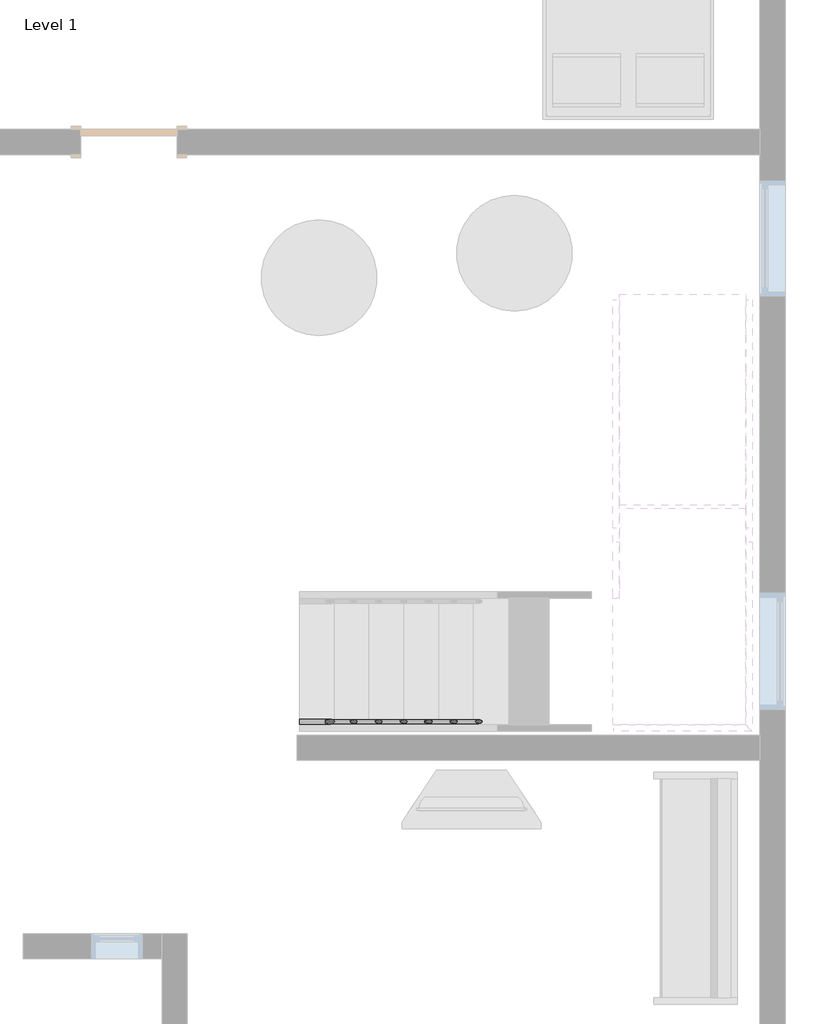
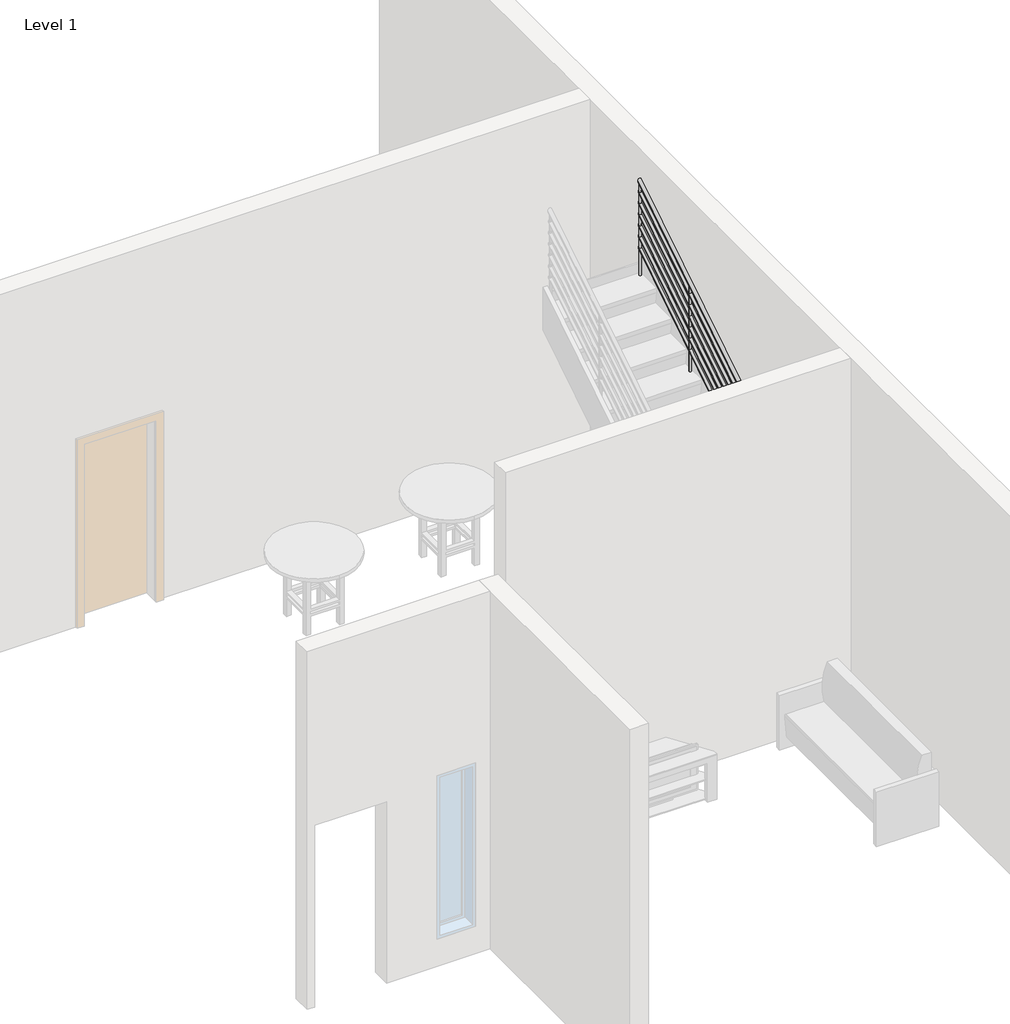
# One storey, part 3 of 4: 1 railing.
"""IFC4 building model written with IfcOpenShell, lengths in millimetres."""

from ifc_helpers import new_model, si_unit, point, frame, frame_2d, origin, place, context, project, spatial, circle_curve, ellipse_curve, trimmed, segment, composite_curve, outline, extrude, element, save
from ifc_brep_helpers import plane_surface, cylinder_surface, advanced_brep

model = new_model("IFC4")

# Units and contexts
model_context = context("Model", 3, world=origin())
ifc_project = project(units=[si_unit("LENGTHUNIT", "METRE", prefix="MILLI")], contexts=[model_context])

# Site, building, storey
site = spatial("IfcSite", under=ifc_project)
building = spatial("IfcBuilding", under=site)
storey = spatial("IfcBuildingStorey", under=building, Name="Level 1", Elevation=0.0)

# Railing
placement = place(None, origin())
element("IfcRailing", 1, ObjectType="900mm Pipe", at=placement, inside=storey, context=model_context, shape_type="SolidModel", body=[
    advanced_brep(
    [(-399.786154, 2752.4262668, 1050.2491997), (-399.786154, 2792.4262668, 1050.2491997), (2081.007299, 2752.4262668, 2619.1304348), (2081.007299, 2792.4262668, 2619.1304348), (3120.6396272, 2752.4262668, 2619.1304348), (3080.6396272, 2792.4262668, 2619.1304348), (3120.6396272, 4184.041917, 2619.1304348), (3080.6396272, 4184.041917, 2619.1304348), (3120.6396272, 6103.248464, 3832.8578953), (3080.6396272, 6103.248464, 3832.8578953)],
    [
        (0, 1, ellipse_curve(frame((-399.786154, 2772.4262668, 1050.2491997), z_axis=(-1.0, 0.0, 0.0), x_axis=(0.0, 0.0, -1.0)), 23.6638438, 20.0)),
        (1, 0, ellipse_curve(frame((-399.786154, 2772.4262668, 1050.2491997), z_axis=(-1.0, 0.0, 0.0), x_axis=(0.0, 0.0, -1.0)), 23.6638438, 20.0)),
        (0, 2),
        (2, 3, ellipse_curve(frame((2081.007299, 2772.4262668, 2619.1304348), z_axis=(-0.9605132043335073, 0.0, -0.2782344053149758), x_axis=(0.2782344053149764, 0.0, -0.9605132043335071)), 20.822202, 20.0)),
        (3, 1),
        (3, 2, ellipse_curve(frame((2081.007299, 2772.4262668, 2619.1304348), z_axis=(-0.9605132043335073, 0.0, -0.2782344053149758), x_axis=(0.2782344053149764, 0.0, -0.9605132043335071)), 20.822202, 20.0)),
        (2, 4),
        (4, 5, ellipse_curve(frame((3100.6396272, 2772.4262668, 2619.1304348), z_axis=(-0.7071067811865493, -0.7071067811865456, 0.0), x_axis=(-0.7071067811865458, 0.7071067811865492, 0.0)), 28.2842712, 20.0)),
        (5, 3),
        (5, 4, ellipse_curve(frame((3100.6396272, 2772.4262668, 2619.1304348), z_axis=(-0.7071067811865493, -0.7071067811865456, 0.0), x_axis=(-0.7071067811865458, 0.7071067811865492, 0.0)), 28.2842712, 20.0)),
        (4, 6),
        (6, 7, ellipse_curve(frame((3100.6396272, 4184.041917, 2619.1304348), z_axis=(0.0, -0.9605132043335073, -0.27823440531497556), x_axis=(0.0, -0.27823440531497573, 0.9605132043335072)), 20.822202, 20.0)),
        (7, 5),
        (7, 6, ellipse_curve(frame((3100.6396272, 4184.041917, 2619.1304348), z_axis=(0.0, -0.9605132043335073, -0.27823440531497556), x_axis=(0.0, -0.27823440531497573, 0.9605132043335072)), 20.822202, 20.0)),
        (8, 9, ellipse_curve(frame((3100.6396272, 6103.248464, 3832.8578953), z_axis=(0.0, 1.0, 0.0), x_axis=(0.0, 0.0, -1.0)), 23.6638438, 20.0)),
        (9, 8, ellipse_curve(frame((3100.6396272, 6103.248464, 3832.8578953), z_axis=(0.0, 1.0, 0.0), x_axis=(0.0, 0.0, -1.0)), 23.6638438, 20.0)),
        (6, 8),
        (9, 7),
    ],
    [
        plane_surface(frame((-399.786154, 2772.4262668, 1073.9130435), z_axis=(-1.0, 0.0, 0.0), x_axis=(0.0, 1.0, 0.0))),
        cylinder_surface(frame((-389.0962412, 2772.4262668, 1057.0096189), z_axis=(-0.8451712313980436, 0.0, -0.5344956404098303), x_axis=(0.0, 1.0, 0.0)), 20.0),
        cylinder_surface(frame((2075.213846, 2772.4262668, 2619.1304348), z_axis=(-1.0, 0.0, 0.0), x_axis=(0.0, 1.0, 0.0)), 20.0),
        cylinder_surface(frame((3100.6396272, 2772.4262668, 2619.1304348), z_axis=(0.0, -1.0, 0.0), x_axis=(-1.0, 0.0, 0.0)), 20.0),
        plane_surface(frame((3100.6396272, 6103.248464, 3856.5217391), z_axis=(0.0, 1.0, 0.0), x_axis=(0.0, 0.0, 1.0))),
        cylinder_surface(frame((3100.6396272, 4188.9383768, 2622.2270102), z_axis=(0.0, -0.8451712313980438, -0.5344956404098301), x_axis=(-1.0, 0.0, 0.0)), 20.0),
    ],
    [
        (0, [[1, 2]]),
        (1, [[-1, 3, 4, 5]]),
        (1, [[-2, -5, 6, -3]]),
        (2, [[-4, 7, 8, 9]]),
        (2, [[-6, -9, 10, -7]]),
        (3, [[-8, 11, 12, 13]]),
        (3, [[-10, -13, 14, -11]]),
        (4, [[15, 16]]),
        (5, [[-12, 17, -16, 18]]),
        (5, [[-14, -18, -15, -17]]),
    ],
),
    advanced_brep(
    [(-399.786154, 2787.4262668, 931.1651606), (-399.786154, 2757.4262668, 931.1651606), (2079.5589357, 2787.4262668, 2499.1304348), (2079.5589357, 2757.4262668, 2499.1304348), (3085.6396272, 2787.4262668, 2499.1304348), (3115.6396272, 2757.4262668, 2499.1304348), (3085.6396272, 4182.5935537, 2499.1304348), (3115.6396272, 4182.5935537, 2499.1304348), (3085.6396272, 6103.248464, 3713.7738563), (3115.6396272, 6103.248464, 3713.7738563)],
    [
        (0, 1, ellipse_curve(frame((-399.786154, 2772.4262668, 931.1651606), z_axis=(-1.0, 0.0, 0.0), x_axis=(0.0, 0.0, -1.0)), 17.7478828, 15.0)),
        (1, 0, ellipse_curve(frame((-399.786154, 2772.4262668, 931.1651606), z_axis=(-1.0, 0.0, 0.0), x_axis=(0.0, 0.0, -1.0)), 17.7478828, 15.0)),
        (0, 2),
        (2, 3, ellipse_curve(frame((2079.5589357, 2772.4262668, 2499.1304348), z_axis=(-0.9605132043335073, 0.0, -0.2782344053149758), x_axis=(0.2782344053149764, 0.0, -0.9605132043335071)), 15.6166515, 15.0)),
        (3, 1),
        (3, 2, ellipse_curve(frame((2079.5589357, 2772.4262668, 2499.1304348), z_axis=(-0.9605132043335073, 0.0, -0.2782344053149758), x_axis=(0.2782344053149764, 0.0, -0.9605132043335071)), 15.6166515, 15.0)),
        (2, 4),
        (4, 5, ellipse_curve(frame((3100.6396272, 2772.4262668, 2499.1304348), z_axis=(-0.7071067811865493, -0.7071067811865456, 0.0), x_axis=(-0.7071067811865458, 0.7071067811865492, 0.0)), 21.2132034, 15.0)),
        (5, 3),
        (5, 4, ellipse_curve(frame((3100.6396272, 2772.4262668, 2499.1304348), z_axis=(-0.7071067811865493, -0.7071067811865456, 0.0), x_axis=(-0.7071067811865458, 0.7071067811865492, 0.0)), 21.2132034, 15.0)),
        (4, 6),
        (6, 7, ellipse_curve(frame((3100.6396272, 4182.5935537, 2499.1304348), z_axis=(0.0, -0.9605132043335073, -0.27823440531497556), x_axis=(0.0, -0.27823440531497573, 0.9605132043335072)), 15.6166515, 15.0)),
        (7, 5),
        (7, 6, ellipse_curve(frame((3100.6396272, 4182.5935537, 2499.1304348), z_axis=(0.0, -0.9605132043335073, -0.27823440531497556), x_axis=(0.0, -0.27823440531497573, 0.9605132043335072)), 15.6166515, 15.0)),
        (8, 9, ellipse_curve(frame((3100.6396272, 6103.248464, 3713.7738563), z_axis=(0.0, 1.0, 0.0), x_axis=(0.0, 0.0, -1.0)), 17.7478828, 15.0)),
        (9, 8, ellipse_curve(frame((3100.6396272, 6103.248464, 3713.7738563), z_axis=(0.0, 1.0, 0.0), x_axis=(0.0, 0.0, -1.0)), 17.7478828, 15.0)),
        (6, 8),
        (9, 7),
    ],
    [
        plane_surface(frame((-399.786154, 2772.4262668, 948.9130435), z_axis=(-1.0, 0.0, 0.0), x_axis=(0.0, 1.0, 0.0))),
        cylinder_surface(frame((-391.7687194, 2772.4262668, 936.235475), z_axis=(-0.8451712313980436, 0.0, -0.5344956404098303), x_axis=(0.0, -1.0, 0.0)), 15.0),
        cylinder_surface(frame((2075.213846, 2772.4262668, 2499.1304348), z_axis=(-1.0, 0.0, 0.0), x_axis=(0.0, -1.0, 0.0)), 15.0),
        cylinder_surface(frame((3100.6396272, 2772.4262668, 2499.1304348), z_axis=(0.0, -1.0, 0.0), x_axis=(1.0, 0.0, 0.0)), 15.0),
        plane_surface(frame((3100.6396272, 6103.248464, 3731.5217391), z_axis=(0.0, 1.0, 0.0), x_axis=(0.0, 0.0, 1.0))),
        cylinder_surface(frame((3100.6396272, 4186.2658986, 2501.4528663), z_axis=(0.0, -0.8451712313980438, -0.5344956404098301), x_axis=(1.0, 0.0, 0.0)), 15.0),
    ],
    [
        (0, [[1, 2]]),
        (1, [[-1, 3, 4, 5]]),
        (1, [[-2, -5, 6, -3]]),
        (2, [[-4, 7, 8, 9]]),
        (2, [[-6, -9, 10, -7]]),
        (3, [[-8, 11, 12, 13]]),
        (3, [[-10, -13, 14, -11]]),
        (4, [[15, 16]]),
        (5, [[-12, 17, -16, 18]]),
        (5, [[-14, -18, -15, -17]]),
    ],
),
    advanced_brep(
    [(-399.786154, 2787.4262668, 806.1651606), (-399.786154, 2757.4262668, 806.1651606), (2079.5589357, 2787.4262668, 2374.1304348), (2079.5589357, 2757.4262668, 2374.1304348), (3085.6396272, 2787.4262668, 2374.1304348), (3115.6396272, 2757.4262668, 2374.1304348), (3085.6396272, 4182.5935537, 2374.1304348), (3115.6396272, 4182.5935537, 2374.1304348), (3085.6396272, 6103.248464, 3588.7738563), (3115.6396272, 6103.248464, 3588.7738563)],
    [
        (0, 1, ellipse_curve(frame((-399.786154, 2772.4262668, 806.1651606), z_axis=(-1.0, 0.0, 0.0), x_axis=(0.0, 0.0, -1.0)), 17.7478828, 15.0)),
        (1, 0, ellipse_curve(frame((-399.786154, 2772.4262668, 806.1651606), z_axis=(-1.0, 0.0, 0.0), x_axis=(0.0, 0.0, -1.0)), 17.7478828, 15.0)),
        (0, 2),
        (2, 3, ellipse_curve(frame((2079.5589357, 2772.4262668, 2374.1304348), z_axis=(-0.9605132043335073, 0.0, -0.2782344053149758), x_axis=(0.2782344053149764, 0.0, -0.9605132043335071)), 15.6166515, 15.0)),
        (3, 1),
        (3, 2, ellipse_curve(frame((2079.5589357, 2772.4262668, 2374.1304348), z_axis=(-0.9605132043335073, 0.0, -0.2782344053149758), x_axis=(0.2782344053149764, 0.0, -0.9605132043335071)), 15.6166515, 15.0)),
        (2, 4),
        (4, 5, ellipse_curve(frame((3100.6396272, 2772.4262668, 2374.1304348), z_axis=(-0.7071067811865493, -0.7071067811865456, 0.0), x_axis=(-0.7071067811865458, 0.7071067811865492, 0.0)), 21.2132034, 15.0)),
        (5, 3),
        (5, 4, ellipse_curve(frame((3100.6396272, 2772.4262668, 2374.1304348), z_axis=(-0.7071067811865493, -0.7071067811865456, 0.0), x_axis=(-0.7071067811865458, 0.7071067811865492, 0.0)), 21.2132034, 15.0)),
        (4, 6),
        (6, 7, ellipse_curve(frame((3100.6396272, 4182.5935537, 2374.1304348), z_axis=(0.0, -0.9605132043335073, -0.27823440531497556), x_axis=(0.0, -0.27823440531497573, 0.9605132043335072)), 15.6166515, 15.0)),
        (7, 5),
        (7, 6, ellipse_curve(frame((3100.6396272, 4182.5935537, 2374.1304348), z_axis=(0.0, -0.9605132043335073, -0.27823440531497556), x_axis=(0.0, -0.27823440531497573, 0.9605132043335072)), 15.6166515, 15.0)),
        (8, 9, ellipse_curve(frame((3100.6396272, 6103.248464, 3588.7738563), z_axis=(0.0, 1.0, 0.0), x_axis=(0.0, 0.0, -1.0)), 17.7478828, 15.0)),
        (9, 8, ellipse_curve(frame((3100.6396272, 6103.248464, 3588.7738563), z_axis=(0.0, 1.0, 0.0), x_axis=(0.0, 0.0, -1.0)), 17.7478828, 15.0)),
        (6, 8),
        (9, 7),
    ],
    [
        plane_surface(frame((-399.786154, 2772.4262668, 823.9130435), z_axis=(-1.0, 0.0, 0.0), x_axis=(0.0, 1.0, 0.0))),
        cylinder_surface(frame((-391.7687194, 2772.4262668, 811.235475), z_axis=(-0.8451712313980436, 0.0, -0.5344956404098303), x_axis=(0.0, -1.0, 0.0)), 15.0),
        cylinder_surface(frame((2075.213846, 2772.4262668, 2374.1304348), z_axis=(-1.0, 0.0, 0.0), x_axis=(0.0, -1.0, 0.0)), 15.0),
        cylinder_surface(frame((3100.6396272, 2772.4262668, 2374.1304348), z_axis=(0.0, -1.0, 0.0), x_axis=(1.0, 0.0, 0.0)), 15.0),
        plane_surface(frame((3100.6396272, 6103.248464, 3606.5217391), z_axis=(0.0, 1.0, 0.0), x_axis=(0.0, 0.0, 1.0))),
        cylinder_surface(frame((3100.6396272, 4186.2658986, 2376.4528663), z_axis=(0.0, -0.8451712313980438, -0.5344956404098301), x_axis=(1.0, 0.0, 0.0)), 15.0),
    ],
    [
        (0, [[1, 2]]),
        (1, [[-1, 3, 4, 5]]),
        (1, [[-2, -5, 6, -3]]),
        (2, [[-4, 7, 8, 9]]),
        (2, [[-6, -9, 10, -7]]),
        (3, [[-8, 11, 12, 13]]),
        (3, [[-10, -13, 14, -11]]),
        (4, [[15, 16]]),
        (5, [[-12, 17, -16, 18]]),
        (5, [[-14, -18, -15, -17]]),
    ],
),
    advanced_brep(
    [(-399.786154, 2787.4262668, 681.1651606), (-399.786154, 2757.4262668, 681.1651606), (2079.5589357, 2787.4262668, 2249.1304348), (2079.5589357, 2757.4262668, 2249.1304348), (3085.6396272, 2787.4262668, 2249.1304348), (3115.6396272, 2757.4262668, 2249.1304348), (3085.6396272, 4182.5935537, 2249.1304348), (3115.6396272, 4182.5935537, 2249.1304348), (3085.6396272, 6103.248464, 3463.7738563), (3115.6396272, 6103.248464, 3463.7738563)],
    [
        (0, 1, ellipse_curve(frame((-399.786154, 2772.4262668, 681.1651606), z_axis=(-1.0, 0.0, 0.0), x_axis=(0.0, 0.0, -1.0)), 17.7478828, 15.0)),
        (1, 0, ellipse_curve(frame((-399.786154, 2772.4262668, 681.1651606), z_axis=(-1.0, 0.0, 0.0), x_axis=(0.0, 0.0, -1.0)), 17.7478828, 15.0)),
        (0, 2),
        (2, 3, ellipse_curve(frame((2079.5589357, 2772.4262668, 2249.1304348), z_axis=(-0.9605132043335073, 0.0, -0.2782344053149758), x_axis=(0.2782344053149764, 0.0, -0.9605132043335071)), 15.6166515, 15.0)),
        (3, 1),
        (3, 2, ellipse_curve(frame((2079.5589357, 2772.4262668, 2249.1304348), z_axis=(-0.9605132043335073, 0.0, -0.2782344053149758), x_axis=(0.2782344053149764, 0.0, -0.9605132043335071)), 15.6166515, 15.0)),
        (2, 4),
        (4, 5, ellipse_curve(frame((3100.6396272, 2772.4262668, 2249.1304348), z_axis=(-0.7071067811865493, -0.7071067811865456, 0.0), x_axis=(-0.7071067811865458, 0.7071067811865492, 0.0)), 21.2132034, 15.0)),
        (5, 3),
        (5, 4, ellipse_curve(frame((3100.6396272, 2772.4262668, 2249.1304348), z_axis=(-0.7071067811865493, -0.7071067811865456, 0.0), x_axis=(-0.7071067811865458, 0.7071067811865492, 0.0)), 21.2132034, 15.0)),
        (4, 6),
        (6, 7, ellipse_curve(frame((3100.6396272, 4182.5935537, 2249.1304348), z_axis=(0.0, -0.9605132043335073, -0.27823440531497545), x_axis=(0.0, -0.27823440531497584, 0.9605132043335073)), 15.6166515, 15.0)),
        (7, 5),
        (7, 6, ellipse_curve(frame((3100.6396272, 4182.5935537, 2249.1304348), z_axis=(0.0, -0.9605132043335073, -0.27823440531497545), x_axis=(0.0, -0.27823440531497584, 0.9605132043335073)), 15.6166515, 15.0)),
        (8, 9, ellipse_curve(frame((3100.6396272, 6103.248464, 3463.7738563), z_axis=(0.0, 1.0, 0.0), x_axis=(0.0, 0.0, -1.0)), 17.7478828, 15.0)),
        (9, 8, ellipse_curve(frame((3100.6396272, 6103.248464, 3463.7738563), z_axis=(0.0, 1.0, 0.0), x_axis=(0.0, 0.0, -1.0)), 17.7478828, 15.0)),
        (6, 8),
        (9, 7),
    ],
    [
        plane_surface(frame((-399.786154, 2772.4262668, 698.9130435), z_axis=(-1.0, 0.0, 0.0), x_axis=(0.0, 1.0, 0.0))),
        cylinder_surface(frame((-391.7687194, 2772.4262668, 686.235475), z_axis=(-0.8451712313980436, 0.0, -0.5344956404098303), x_axis=(0.0, -1.0, 0.0)), 15.0),
        cylinder_surface(frame((2075.213846, 2772.4262668, 2249.1304348), z_axis=(-1.0, 0.0, 0.0), x_axis=(0.0, -1.0, 0.0)), 15.0),
        cylinder_surface(frame((3100.6396272, 2772.4262668, 2249.1304348), z_axis=(0.0, -1.0, 0.0), x_axis=(1.0, 0.0, 0.0)), 15.0),
        plane_surface(frame((3100.6396272, 6103.248464, 3481.5217391), z_axis=(0.0, 1.0, 0.0), x_axis=(0.0, 0.0, 1.0))),
        cylinder_surface(frame((3100.6396272, 4186.2658986, 2251.4528663), z_axis=(0.0, -0.845171231398044, -0.5344956404098299), x_axis=(1.0, 0.0, 0.0)), 15.0),
    ],
    [
        (0, [[1, 2]]),
        (1, [[-1, 3, 4, 5]]),
        (1, [[-2, -5, 6, -3]]),
        (2, [[-4, 7, 8, 9]]),
        (2, [[-6, -9, 10, -7]]),
        (3, [[-8, 11, 12, 13]]),
        (3, [[-10, -13, 14, -11]]),
        (4, [[15, 16]]),
        (5, [[-12, 17, -16, 18]]),
        (5, [[-14, -18, -15, -17]]),
    ],
),
    advanced_brep(
    [(-399.786154, 2787.4262668, 556.1651606), (-399.786154, 2757.4262668, 556.1651606), (2079.5589357, 2787.4262668, 2124.1304348), (2079.5589357, 2757.4262668, 2124.1304348), (3085.6396272, 2787.4262668, 2124.1304348), (3115.6396272, 2757.4262668, 2124.1304348), (3085.6396272, 4182.5935537, 2124.1304348), (3115.6396272, 4182.5935537, 2124.1304348), (3085.6396272, 6103.248464, 3338.7738563), (3115.6396272, 6103.248464, 3338.7738563)],
    [
        (0, 1, ellipse_curve(frame((-399.786154, 2772.4262668, 556.1651606), z_axis=(-1.0, 0.0, 0.0), x_axis=(0.0, 0.0, -1.0)), 17.7478828, 15.0)),
        (1, 0, ellipse_curve(frame((-399.786154, 2772.4262668, 556.1651606), z_axis=(-1.0, 0.0, 0.0), x_axis=(0.0, 0.0, -1.0)), 17.7478828, 15.0)),
        (0, 2),
        (2, 3, ellipse_curve(frame((2079.5589357, 2772.4262668, 2124.1304348), z_axis=(-0.9605132043335073, 0.0, -0.2782344053149758), x_axis=(0.2782344053149764, 0.0, -0.9605132043335071)), 15.6166515, 15.0)),
        (3, 1),
        (3, 2, ellipse_curve(frame((2079.5589357, 2772.4262668, 2124.1304348), z_axis=(-0.9605132043335073, 0.0, -0.2782344053149758), x_axis=(0.2782344053149764, 0.0, -0.9605132043335071)), 15.6166515, 15.0)),
        (2, 4),
        (4, 5, ellipse_curve(frame((3100.6396272, 2772.4262668, 2124.1304348), z_axis=(-0.7071067811865493, -0.7071067811865456, 0.0), x_axis=(-0.7071067811865458, 0.7071067811865492, 0.0)), 21.2132034, 15.0)),
        (5, 3),
        (5, 4, ellipse_curve(frame((3100.6396272, 2772.4262668, 2124.1304348), z_axis=(-0.7071067811865493, -0.7071067811865456, 0.0), x_axis=(-0.7071067811865458, 0.7071067811865492, 0.0)), 21.2132034, 15.0)),
        (4, 6),
        (6, 7, ellipse_curve(frame((3100.6396272, 4182.5935537, 2124.1304348), z_axis=(0.0, -0.9605132043335073, -0.27823440531497556), x_axis=(0.0, -0.27823440531497573, 0.9605132043335072)), 15.6166515, 15.0)),
        (7, 5),
        (7, 6, ellipse_curve(frame((3100.6396272, 4182.5935537, 2124.1304348), z_axis=(0.0, -0.9605132043335073, -0.27823440531497556), x_axis=(0.0, -0.27823440531497573, 0.9605132043335072)), 15.6166515, 15.0)),
        (8, 9, ellipse_curve(frame((3100.6396272, 6103.248464, 3338.7738563), z_axis=(0.0, 1.0, 0.0), x_axis=(0.0, 0.0, -1.0)), 17.7478828, 15.0)),
        (9, 8, ellipse_curve(frame((3100.6396272, 6103.248464, 3338.7738563), z_axis=(0.0, 1.0, 0.0), x_axis=(0.0, 0.0, -1.0)), 17.7478828, 15.0)),
        (6, 8),
        (9, 7),
    ],
    [
        plane_surface(frame((-399.786154, 2772.4262668, 573.9130435), z_axis=(-1.0, 0.0, 0.0), x_axis=(0.0, 1.0, 0.0))),
        cylinder_surface(frame((-391.7687194, 2772.4262668, 561.235475), z_axis=(-0.8451712313980436, 0.0, -0.5344956404098303), x_axis=(0.0, -1.0, 0.0)), 15.0),
        cylinder_surface(frame((2075.213846, 2772.4262668, 2124.1304348), z_axis=(-1.0, 0.0, 0.0), x_axis=(0.0, -1.0, 0.0)), 15.0),
        cylinder_surface(frame((3100.6396272, 2772.4262668, 2124.1304348), z_axis=(0.0, -1.0, 0.0), x_axis=(1.0, 0.0, 0.0)), 15.0),
        plane_surface(frame((3100.6396272, 6103.248464, 3356.5217391), z_axis=(0.0, 1.0, 0.0), x_axis=(0.0, 0.0, 1.0))),
        cylinder_surface(frame((3100.6396272, 4186.2658986, 2126.4528663), z_axis=(0.0, -0.8451712313980438, -0.5344956404098301), x_axis=(1.0, 0.0, 0.0)), 15.0),
    ],
    [
        (0, [[1, 2]]),
        (1, [[-1, 3, 4, 5]]),
        (1, [[-2, -5, 6, -3]]),
        (2, [[-4, 7, 8, 9]]),
        (2, [[-6, -9, 10, -7]]),
        (3, [[-8, 11, 12, 13]]),
        (3, [[-10, -13, 14, -11]]),
        (4, [[15, 16]]),
        (5, [[-12, 17, -16, 18]]),
        (5, [[-14, -18, -15, -17]]),
    ],
),
    advanced_brep(
    [(-399.786154, 2787.4262668, 431.1651606), (-399.786154, 2757.4262668, 431.1651606), (2079.5589357, 2787.4262668, 1999.1304348), (2079.5589357, 2757.4262668, 1999.1304348), (3085.6396272, 2787.4262668, 1999.1304348), (3115.6396272, 2757.4262668, 1999.1304348), (3085.6396272, 4182.5935537, 1999.1304348), (3115.6396272, 4182.5935537, 1999.1304348), (3085.6396272, 6103.248464, 3213.7738563), (3115.6396272, 6103.248464, 3213.7738563)],
    [
        (0, 1, ellipse_curve(frame((-399.786154, 2772.4262668, 431.1651606), z_axis=(-1.0, 0.0, 0.0), x_axis=(0.0, 0.0, -1.0)), 17.7478828, 15.0)),
        (1, 0, ellipse_curve(frame((-399.786154, 2772.4262668, 431.1651606), z_axis=(-1.0, 0.0, 0.0), x_axis=(0.0, 0.0, -1.0)), 17.7478828, 15.0)),
        (0, 2),
        (2, 3, ellipse_curve(frame((2079.5589357, 2772.4262668, 1999.1304348), z_axis=(-0.9605132043335073, 0.0, -0.2782344053149758), x_axis=(0.2782344053149764, 0.0, -0.9605132043335071)), 15.6166515, 15.0)),
        (3, 1),
        (3, 2, ellipse_curve(frame((2079.5589357, 2772.4262668, 1999.1304348), z_axis=(-0.9605132043335073, 0.0, -0.2782344053149758), x_axis=(0.2782344053149764, 0.0, -0.9605132043335071)), 15.6166515, 15.0)),
        (2, 4),
        (4, 5, ellipse_curve(frame((3100.6396272, 2772.4262668, 1999.1304348), z_axis=(-0.7071067811865493, -0.7071067811865456, 0.0), x_axis=(-0.7071067811865458, 0.7071067811865492, 0.0)), 21.2132034, 15.0)),
        (5, 3),
        (5, 4, ellipse_curve(frame((3100.6396272, 2772.4262668, 1999.1304348), z_axis=(-0.7071067811865493, -0.7071067811865456, 0.0), x_axis=(-0.7071067811865458, 0.7071067811865492, 0.0)), 21.2132034, 15.0)),
        (4, 6),
        (6, 7, ellipse_curve(frame((3100.6396272, 4182.5935537, 1999.1304348), z_axis=(0.0, -0.9605132043335072, -0.27823440531497556), x_axis=(0.0, -0.2782344053149761, 0.9605132043335072)), 15.6166515, 15.0)),
        (7, 5),
        (7, 6, ellipse_curve(frame((3100.6396272, 4182.5935537, 1999.1304348), z_axis=(0.0, -0.9605132043335072, -0.27823440531497556), x_axis=(0.0, -0.2782344053149761, 0.9605132043335072)), 15.6166515, 15.0)),
        (8, 9, ellipse_curve(frame((3100.6396272, 6103.248464, 3213.7738563), z_axis=(0.0, 1.0, 0.0), x_axis=(0.0, 0.0, -1.0)), 17.7478828, 15.0)),
        (9, 8, ellipse_curve(frame((3100.6396272, 6103.248464, 3213.7738563), z_axis=(0.0, 1.0, 0.0), x_axis=(0.0, 0.0, -1.0)), 17.7478828, 15.0)),
        (6, 8),
        (9, 7),
    ],
    [
        plane_surface(frame((-399.786154, 2772.4262668, 448.9130435), z_axis=(-1.0, 0.0, 0.0), x_axis=(0.0, 1.0, 0.0))),
        cylinder_surface(frame((-391.7687194, 2772.4262668, 436.235475), z_axis=(-0.8451712313980436, 0.0, -0.5344956404098303), x_axis=(0.0, -1.0, 0.0)), 15.0),
        cylinder_surface(frame((2075.213846, 2772.4262668, 1999.1304348), z_axis=(-1.0, 0.0, 0.0), x_axis=(0.0, -1.0, 0.0)), 15.0),
        cylinder_surface(frame((3100.6396272, 2772.4262668, 1999.1304348), z_axis=(0.0, -1.0, 0.0), x_axis=(1.0, 0.0, 0.0)), 15.0),
        plane_surface(frame((3100.6396272, 6103.248464, 3231.5217391), z_axis=(0.0, 1.0, 0.0), x_axis=(0.0, 0.0, 1.0))),
        cylinder_surface(frame((3100.6396272, 4186.2658986, 2001.4528663), z_axis=(0.0, -0.8451712313980437, -0.5344956404098301), x_axis=(1.0, 0.0, 0.0)), 15.0),
    ],
    [
        (0, [[1, 2]]),
        (1, [[-1, 3, 4, 5]]),
        (1, [[-2, -5, 6, -3]]),
        (2, [[-4, 7, 8, 9]]),
        (2, [[-6, -9, 10, -7]]),
        (3, [[-8, 11, 12, 13]]),
        (3, [[-10, -13, 14, -11]]),
        (4, [[15, 16]]),
        (5, [[-12, 17, -16, 18]]),
        (5, [[-14, -18, -15, -17]]),
    ],
),
    advanced_brep(
    [(-399.786154, 2787.4262668, 306.1651606), (-399.786154, 2757.4262668, 306.1651606), (2079.5589357, 2787.4262668, 1874.1304348), (2079.5589357, 2757.4262668, 1874.1304348), (3085.6396272, 2787.4262668, 1874.1304348), (3115.6396272, 2757.4262668, 1874.1304348), (3085.6396272, 4182.5935537, 1874.1304348), (3115.6396272, 4182.5935537, 1874.1304348), (3085.6396272, 6103.248464, 3088.7738563), (3115.6396272, 6103.248464, 3088.7738563)],
    [
        (0, 1, ellipse_curve(frame((-399.786154, 2772.4262668, 306.1651606), z_axis=(-1.0, 0.0, 0.0), x_axis=(0.0, 0.0, -1.0)), 17.7478828, 15.0)),
        (1, 0, ellipse_curve(frame((-399.786154, 2772.4262668, 306.1651606), z_axis=(-1.0, 0.0, 0.0), x_axis=(0.0, 0.0, -1.0)), 17.7478828, 15.0)),
        (0, 2),
        (2, 3, ellipse_curve(frame((2079.5589357, 2772.4262668, 1874.1304348), z_axis=(-0.9605132043335073, 0.0, -0.2782344053149758), x_axis=(0.2782344053149764, 0.0, -0.9605132043335071)), 15.6166515, 15.0)),
        (3, 1),
        (3, 2, ellipse_curve(frame((2079.5589357, 2772.4262668, 1874.1304348), z_axis=(-0.9605132043335073, 0.0, -0.2782344053149758), x_axis=(0.2782344053149764, 0.0, -0.9605132043335071)), 15.6166515, 15.0)),
        (2, 4),
        (4, 5, ellipse_curve(frame((3100.6396272, 2772.4262668, 1874.1304348), z_axis=(-0.7071067811865493, -0.7071067811865456, 0.0), x_axis=(-0.7071067811865458, 0.7071067811865492, 0.0)), 21.2132034, 15.0)),
        (5, 3),
        (5, 4, ellipse_curve(frame((3100.6396272, 2772.4262668, 1874.1304348), z_axis=(-0.7071067811865493, -0.7071067811865456, 0.0), x_axis=(-0.7071067811865458, 0.7071067811865492, 0.0)), 21.2132034, 15.0)),
        (4, 6),
        (6, 7, ellipse_curve(frame((3100.6396272, 4182.5935537, 1874.1304348), z_axis=(0.0, -0.9605132043335073, -0.27823440531497556), x_axis=(0.0, -0.27823440531497573, 0.9605132043335072)), 15.6166515, 15.0)),
        (7, 5),
        (7, 6, ellipse_curve(frame((3100.6396272, 4182.5935537, 1874.1304348), z_axis=(0.0, -0.9605132043335073, -0.27823440531497556), x_axis=(0.0, -0.27823440531497573, 0.9605132043335072)), 15.6166515, 15.0)),
        (8, 9, ellipse_curve(frame((3100.6396272, 6103.248464, 3088.7738563), z_axis=(0.0, 1.0, 0.0), x_axis=(0.0, 0.0, -1.0)), 17.7478828, 15.0)),
        (9, 8, ellipse_curve(frame((3100.6396272, 6103.248464, 3088.7738563), z_axis=(0.0, 1.0, 0.0), x_axis=(0.0, 0.0, -1.0)), 17.7478828, 15.0)),
        (6, 8),
        (9, 7),
    ],
    [
        plane_surface(frame((-399.786154, 2772.4262668, 323.9130435), z_axis=(-1.0, 0.0, 0.0), x_axis=(0.0, 1.0, 0.0))),
        cylinder_surface(frame((-391.7687194, 2772.4262668, 311.235475), z_axis=(-0.8451712313980436, 0.0, -0.5344956404098303), x_axis=(0.0, -1.0, 0.0)), 15.0),
        cylinder_surface(frame((2075.213846, 2772.4262668, 1874.1304348), z_axis=(-1.0, 0.0, 0.0), x_axis=(0.0, -1.0, 0.0)), 15.0),
        cylinder_surface(frame((3100.6396272, 2772.4262668, 1874.1304348), z_axis=(0.0, -1.0, 0.0), x_axis=(1.0, 0.0, 0.0)), 15.0),
        plane_surface(frame((3100.6396272, 6103.248464, 3106.5217391), z_axis=(0.0, 1.0, 0.0), x_axis=(0.0, 0.0, 1.0))),
        cylinder_surface(frame((3100.6396272, 4186.2658986, 1876.4528663), z_axis=(0.0, -0.8451712313980438, -0.5344956404098301), x_axis=(1.0, 0.0, 0.0)), 15.0),
    ],
    [
        (0, [[1, 2]]),
        (1, [[-1, 3, 4, 5]]),
        (1, [[-2, -5, 6, -3]]),
        (2, [[-4, 7, 8, 9]]),
        (2, [[-6, -9, 10, -7]]),
        (3, [[-8, 11, 12, 13]]),
        (3, [[-10, -13, 14, -11]]),
        (4, [[15, 16]]),
        (5, [[-12, 17, -16, 18]]),
        (5, [[-14, -18, -15, -17]]),
    ],
),
    advanced_brep(
    [(3113.1396272, 5178.248464, 3224.2138144), (3113.1396272, 5178.248464, 2260.8695652), (3088.1396272, 5178.248464, 2260.8695652), (3088.1396272, 5178.248464, 3224.2138144)],
    [
        (0, 1),
        (1, 2, circle_curve(frame((3100.6396272, 5178.248464, 2260.8695652), z_axis=(0.0, 0.0, 1.0), x_axis=(-1.0, 0.0, 0.0)), 12.5)),
        (2, 3),
        (3, 0, ellipse_curve(frame((3100.6396272, 5178.248464, 3224.2138144), z_axis=(0.0, 0.5344956404098302, -0.8451712313980437), x_axis=(0.0, 0.8451712313980437, 0.53449564040983)), 14.7899024, 12.5)),
        (0, 3, ellipse_curve(frame((3100.6396272, 5178.248464, 3224.2138144), z_axis=(0.0, 0.5344956404098302, -0.8451712313980437), x_axis=(0.0, 0.8451712313980437, 0.53449564040983)), 14.7899024, 12.5)),
        (2, 1, circle_curve(frame((3100.6396272, 5178.248464, 2260.8695652), z_axis=(0.0, 0.0, 1.0), x_axis=(-1.0, 0.0, 0.0)), 12.5)),
    ],
    [
        cylinder_surface(frame((3100.6396272, 5178.248464, 2160.8695652), z_axis=(0.0, 0.0, 1.0), x_axis=(-1.0, 0.0, 0.0)), 12.5),
        plane_surface(frame((3075.6396272, 5203.248464, 3240.0240911), z_axis=(0.0, -0.5344956404098302, 0.8451712313980437), x_axis=(1.0, 0.0, 0.0))),
        plane_surface(frame((3075.6396272, 5153.248464, 2260.8695652), z_axis=(0.0, 0.0, -1.0), x_axis=(1.0, 0.0, 0.0))),
    ],
    [
        (0, [[1, 2, 3, 4]]),
        (0, [[-1, 5, -3, 6]]),
        (1, [[-4, -5]]),
        (2, [[-2, -6]]),
    ],
),
    extrude(outline(composite_curve([segment(trimmed(circle_curve(frame_2d((3100.6396272, 3772.4262668)), 12.5), [point((3088.1396272, 3772.4262668))], [point((3113.1396272, 3772.4262668))], False, "CARTESIAN"), True, "CONTINUOUS"), segment(trimmed(circle_curve(frame_2d((3100.6396272, 3772.4262668)), 12.5), [point((3113.1396272, 3772.4262668))], [point((3088.1396272, 3772.4262668))], False, "CARTESIAN"), True, "CONTINUOUS")], self_intersect=False)), frame((0.0, 0.0, 1739.1304348), z_axis=(0.0, 0.0, 1.0), x_axis=(1.0, 0.0, 0.0)), (0.0, 0.0, 1.0), 860.0),
    extrude(outline(composite_curve([segment(trimmed(circle_curve(frame_2d((3075.213846, 2772.4262668)), 12.5), [point((3075.213846, 2784.9262668))], [point((3075.213846, 2759.9262668))], False, "CARTESIAN"), True, "CONTINUOUS"), segment(trimmed(circle_curve(frame_2d((3075.213846, 2772.4262668)), 12.5), [point((3075.213846, 2759.9262668))], [point((3075.213846, 2784.9262668))], False, "CARTESIAN"), True, "CONTINUOUS")], self_intersect=False)), frame((0.0, 0.0, 1739.1304348), z_axis=(0.0, 0.0, 1.0), x_axis=(1.0, 0.0, 0.0)), (0.0, 0.0, 1.0), 860.0),
    advanced_brep(
    [(1600.213846, 2759.9262668, 2291.4074903), (1600.213846, 2759.9262668, 1391.3043478), (1600.213846, 2784.9262668, 1391.3043478), (1600.213846, 2784.9262668, 2291.4074903)],
    [
        (0, 1),
        (1, 2, circle_curve(frame((1600.213846, 2772.4262668, 1391.3043478), z_axis=(0.0, 0.0, 1.0), x_axis=(0.0, 1.0, 0.0)), 12.5)),
        (2, 3),
        (3, 0, ellipse_curve(frame((1600.213846, 2772.4262668, 2291.4074903), z_axis=(0.5344956404098302, 0.0, -0.8451712313980437), x_axis=(0.8451712313980437, 0.0, 0.53449564040983)), 14.7899024, 12.5)),
        (0, 3, ellipse_curve(frame((1600.213846, 2772.4262668, 2291.4074903), z_axis=(0.5344956404098302, 0.0, -0.8451712313980437), x_axis=(0.8451712313980437, 0.0, 0.53449564040983)), 14.7899024, 12.5)),
        (2, 1, circle_curve(frame((1600.213846, 2772.4262668, 1391.3043478), z_axis=(0.0, 0.0, 1.0), x_axis=(0.0, 1.0, 0.0)), 12.5)),
    ],
    [
        cylinder_surface(frame((1600.213846, 2772.4262668, 1291.3043478), z_axis=(0.0, 0.0, 1.0), x_axis=(0.0, 1.0, 0.0)), 12.5),
        plane_surface(frame((1625.213846, 2797.4262668, 2307.217767), z_axis=(-0.5344956404098302, 0.0, 0.8451712313980437), x_axis=(0.0, -1.0, 0.0))),
        plane_surface(frame((1575.213846, 2797.4262668, 1391.3043478), z_axis=(0.0, 0.0, -1.0), x_axis=(0.0, -1.0, 0.0))),
    ],
    [
        (0, [[1, 2, 3, 4]]),
        (0, [[-1, 5, -3, 6]]),
        (1, [[-4, -5]]),
        (2, [[-2, -6]]),
    ],
),
    advanced_brep(
    [(600.213846, 2759.9262668, 1658.9964231), (600.213846, 2759.9262668, 695.6521739), (600.213846, 2784.9262668, 695.6521739), (600.213846, 2784.9262668, 1658.9964231)],
    [
        (0, 1),
        (1, 2, circle_curve(frame((600.213846, 2772.4262668, 695.6521739), z_axis=(0.0, 0.0, 1.0), x_axis=(0.0, 1.0, 0.0)), 12.5)),
        (2, 3),
        (3, 0, ellipse_curve(frame((600.213846, 2772.4262668, 1658.9964231), z_axis=(0.5344956404098302, 0.0, -0.8451712313980437), x_axis=(0.8451712313980437, 0.0, 0.53449564040983)), 14.7899024, 12.5)),
        (0, 3, ellipse_curve(frame((600.213846, 2772.4262668, 1658.9964231), z_axis=(0.5344956404098302, 0.0, -0.8451712313980437), x_axis=(0.8451712313980437, 0.0, 0.53449564040983)), 14.7899024, 12.5)),
        (2, 1, circle_curve(frame((600.213846, 2772.4262668, 695.6521739), z_axis=(0.0, 0.0, 1.0), x_axis=(0.0, 1.0, 0.0)), 12.5)),
    ],
    [
        cylinder_surface(frame((600.213846, 2772.4262668, 595.6521739), z_axis=(0.0, 0.0, 1.0), x_axis=(0.0, 1.0, 0.0)), 12.5),
        plane_surface(frame((625.213846, 2797.4262668, 1674.8066998), z_axis=(-0.5344956404098302, 0.0, 0.8451712313980437), x_axis=(0.0, -1.0, 0.0))),
        plane_surface(frame((575.213846, 2797.4262668, 695.6521739), z_axis=(0.0, 0.0, -1.0), x_axis=(0.0, -1.0, 0.0))),
    ],
    [
        (0, [[1, 2, 3, 4]]),
        (0, [[-1, 5, -3, 6]]),
        (1, [[-4, -5]]),
        (2, [[-2, -6]]),
    ],
),
    extrude(outline(composite_curve([segment(trimmed(circle_curve(frame_2d((3100.6396272, 4178.248464)), 12.5), [point((3088.1396272, 4178.248464))], [point((3113.1396272, 4178.248464))], False, "CARTESIAN"), True, "CONTINUOUS"), segment(trimmed(circle_curve(frame_2d((3100.6396272, 4178.248464)), 12.5), [point((3113.1396272, 4178.248464))], [point((3088.1396272, 4178.248464))], False, "CARTESIAN"), True, "CONTINUOUS")], self_intersect=False)), frame((0.0, 0.0, 1739.1304348), z_axis=(0.0, 0.0, 1.0), x_axis=(1.0, 0.0, 0.0)), (0.0, 0.0, 1.0), 860.0),
    extrude(outline(composite_curve([segment(trimmed(circle_curve(frame_2d((3100.6396272, 2772.4262668)), 12.5), [point((3100.6396272, 2784.9262668))], [point((3100.6396272, 2759.9262668))], False, "CARTESIAN"), True, "CONTINUOUS"), segment(trimmed(circle_curve(frame_2d((3100.6396272, 2772.4262668)), 12.5), [point((3100.6396272, 2759.9262668))], [point((3100.6396272, 2784.9262668))], False, "CARTESIAN"), True, "CONTINUOUS")], self_intersect=False)), frame((0.0, 0.0, 1739.1304348), z_axis=(0.0, 0.0, 1.0), x_axis=(1.0, 0.0, 0.0)), (0.0, 0.0, 1.0), 860.0),
    advanced_brep(
    [(2075.213846, 2759.9262668, 2591.8027472), (2075.213846, 2759.9262668, 1739.1304348), (2075.213846, 2784.9262668, 1739.1304348), (2075.213846, 2784.9262668, 2591.8027472)],
    [
        (0, 1),
        (1, 2, circle_curve(frame((2075.213846, 2772.4262668, 1739.1304348), z_axis=(0.0, 0.0, 1.0), x_axis=(0.0, 1.0, 0.0)), 12.5)),
        (2, 3),
        (3, 0, ellipse_curve(frame((2075.213846, 2772.4262668, 2591.8027472), z_axis=(0.5344956404098302, 0.0, -0.8451712313980437), x_axis=(0.8451712313980437, 0.0, 0.53449564040983)), 14.7899024, 12.5)),
        (0, 3, ellipse_curve(frame((2075.213846, 2772.4262668, 2591.8027472), z_axis=(0.5344956404098302, 0.0, -0.8451712313980437), x_axis=(0.8451712313980437, 0.0, 0.53449564040983)), 14.7899024, 12.5)),
        (2, 1, circle_curve(frame((2075.213846, 2772.4262668, 1739.1304348), z_axis=(0.0, 0.0, 1.0), x_axis=(0.0, 1.0, 0.0)), 12.5)),
    ],
    [
        cylinder_surface(frame((2075.213846, 2772.4262668, 1639.1304348), z_axis=(0.0, 0.0, 1.0), x_axis=(0.0, 1.0, 0.0)), 12.5),
        plane_surface(frame((2100.213846, 2797.4262668, 2607.6130239), z_axis=(-0.5344956404098302, 0.0, 0.8451712313980437), x_axis=(0.0, -1.0, 0.0))),
        plane_surface(frame((2050.213846, 2797.4262668, 1739.1304348), z_axis=(0.0, 0.0, -1.0), x_axis=(0.0, -1.0, 0.0))),
    ],
    [
        (0, [[1, 2, 3, 4]]),
        (0, [[-1, 5, -3, 6]]),
        (1, [[-4, -5]]),
        (2, [[-2, -6]]),
    ],
),
    advanced_brep(
    [(3113.1396272, 6090.748464, 3801.2889132), (3113.1396272, 6090.748464, 2782.6086957), (3088.1396272, 6090.748464, 2782.6086957), (3088.1396272, 6090.748464, 3801.2889132)],
    [
        (0, 1),
        (1, 2, circle_curve(frame((3100.6396272, 6090.748464, 2782.6086957), z_axis=(0.0, 0.0, 1.0), x_axis=(-1.0, 0.0, 0.0)), 12.5)),
        (2, 3),
        (3, 0, ellipse_curve(frame((3100.6396272, 6090.748464, 3801.2889132), z_axis=(0.0, 0.5344956404098302, -0.8451712313980437), x_axis=(0.0, 0.8451712313980437, 0.53449564040983)), 14.7899024, 12.5)),
        (0, 3, ellipse_curve(frame((3100.6396272, 6090.748464, 3801.2889132), z_axis=(0.0, 0.5344956404098302, -0.8451712313980437), x_axis=(0.0, 0.8451712313980437, 0.53449564040983)), 14.7899024, 12.5)),
        (2, 1, circle_curve(frame((3100.6396272, 6090.748464, 2782.6086957), z_axis=(0.0, 0.0, 1.0), x_axis=(-1.0, 0.0, 0.0)), 12.5)),
    ],
    [
        cylinder_surface(frame((3100.6396272, 6090.748464, 2682.6086957), z_axis=(0.0, 0.0, 1.0), x_axis=(-1.0, 0.0, 0.0)), 12.5),
        plane_surface(frame((3075.6396272, 6115.748464, 3817.0991899), z_axis=(0.0, -0.5344956404098302, 0.8451712313980437), x_axis=(1.0, 0.0, 0.0))),
        plane_surface(frame((3075.6396272, 6065.748464, 2782.6086957), z_axis=(0.0, 0.0, -1.0), x_axis=(1.0, 0.0, 0.0))),
    ],
    [
        (0, [[1, 2, 3, 4]]),
        (0, [[-1, 5, -3, 6]]),
        (1, [[-4, -5]]),
        (2, [[-2, -6]]),
    ],
),
    advanced_brep(
    [(-387.286154, 2759.9262668, 1034.4904942), (-387.286154, 2759.9262668, 173.9130435), (-387.286154, 2784.9262668, 173.9130435), (-387.286154, 2784.9262668, 1034.4904942)],
    [
        (0, 1),
        (1, 2, circle_curve(frame((-387.286154, 2772.4262668, 173.9130435), z_axis=(0.0, 0.0, 1.0), x_axis=(0.0, 1.0, 0.0)), 12.5)),
        (2, 3),
        (3, 0, ellipse_curve(frame((-387.286154, 2772.4262668, 1034.4904942), z_axis=(0.5344956404098302, 0.0, -0.8451712313980437), x_axis=(0.8451712313980437, 0.0, 0.53449564040983)), 14.7899024, 12.5)),
        (0, 3, ellipse_curve(frame((-387.286154, 2772.4262668, 1034.4904942), z_axis=(0.5344956404098302, 0.0, -0.8451712313980437), x_axis=(0.8451712313980437, 0.0, 0.53449564040983)), 14.7899024, 12.5)),
        (2, 1, circle_curve(frame((-387.286154, 2772.4262668, 173.9130435), z_axis=(0.0, 0.0, 1.0), x_axis=(0.0, 1.0, 0.0)), 12.5)),
    ],
    [
        cylinder_surface(frame((-387.286154, 2772.4262668, 73.9130435), z_axis=(0.0, 0.0, 1.0), x_axis=(0.0, 1.0, 0.0)), 12.5),
        plane_surface(frame((-362.286154, 2797.4262668, 1050.3007709), z_axis=(-0.5344956404098302, 0.0, 0.8451712313980437), x_axis=(0.0, -1.0, 0.0))),
        plane_surface(frame((-412.286154, 2797.4262668, 173.9130435), z_axis=(0.0, 0.0, -1.0), x_axis=(0.0, -1.0, 0.0))),
    ],
    [
        (0, [[1, 2, 3, 4]]),
        (0, [[-1, 5, -3, 6]]),
        (1, [[-4, -5]]),
        (2, [[-2, -6]]),
    ],
),
])

save(model, "model.ifc")

# Revit data of these elements
# Type "900mm Pipe"
#   built-in parameter 1008612 = 0.019685 (stored number, unit not read)
#   built-in parameter 1008611 = 0.0984252 (stored number, unit not read)
#   built-in parameter 1008609 = 6.56168 (stored number, unit not read)
#   built-in parameter 1008604 = 0.19685 (stored number, unit not read)
#   built-in parameter 1008603 = 0.164042 (stored number, unit not read)
#   Railing Height = 2' - 11.43307"
#   built-in parameter 1008630 = 2
#   built-in parameter 1008610 = 2
#   built-in parameter 1008605 = 1
#   built-in parameter 1008618 = M_Baluster - Round : 25mm
# Element 1 (IfcRailing, "900mm Pipe")
#   Phase Created = New Construction
